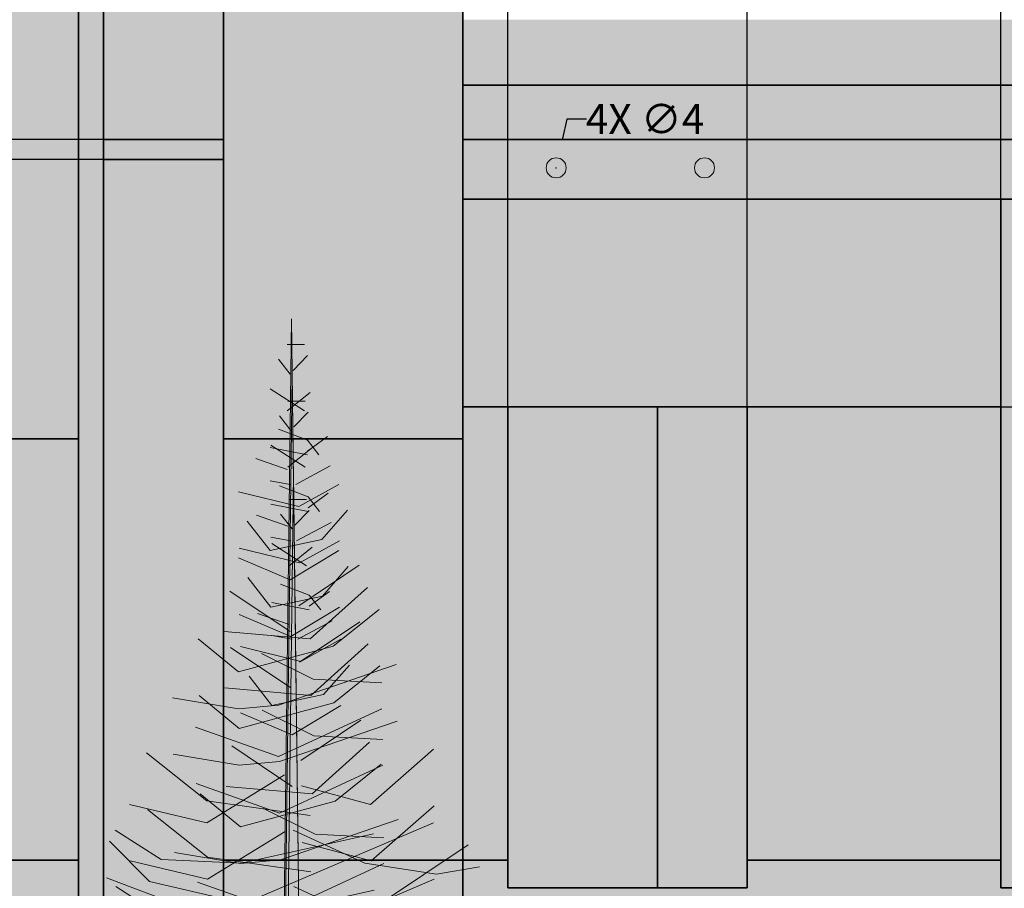
# Model space of a CAD drawing. Units: inches. Extents: x 221 to 874, y 171 to 738.
# Tile 6 of 11: x 452 to 650, y 281 to 455. Entities that reach past the tile are written whole.
import ezdxf

# ---------------------------------------------------------------- set-up
doc = ezdxf.new("R2010")
doc.units = ezdxf.units.IN
doc.header["$MEASUREMENT"] = 0
for name, color, linetype, lineweight in [('A-ANNO-DIMS', 2, 'Continuous', 18), ('A-ELEV', 7, 'Continuous', 35), ('A-ELEV-PATT', 8, 'Continuous', 13), ('E-LITE', 2, 'Continuous', 18), ('L-PLNT', 3, 'Continuous', 13)]:
    doc.layers.add(name, color=color, linetype=linetype, lineweight=lineweight)
doc.styles.get("Standard").update_dxf_attribs({"font": 'arial.ttf'})
doc.dimstyles.get("Standard").update_dxf_attribs({"dimtxt": 6, "dimasz": 4, "dimexe": 0.18, "dimexo": 0.0625, "dimgap": 0.09, "dimtad": 0, "dimtih": 1, "dimtoh": 1, "dimdec": 0, "dimzin": 0, "dimdsep": 46, "dimlunit": 3, "dimtxsty": 'Standard', "dimcen": 0.09, "dimadec": 0, "dimazin": 0, "dimtfac": 1, "dimtdec": 0, "dimtofl": 0, "dimtmove": 0, "dimatfit": 3, "dimfxl": 1, "dimtolj": 1, "dimtzin": 0, "dimarcsym": 0})

# ---------------------------------------------------------------- blocks, each defined once
blk = doc.blocks.new('*D21')
at = {"layer": 'A-ANNO-DIMS', "color": 0, "lineweight": -2, "transparency": 16777216}
for p, q in [((541.14, 706.72), (833.01, 706.72)), ((832.83, 702.72), (832.83, 457.87)), ((832.83, 206.72), (832.83, 451.56)), ((805.14, 202.72), (833.01, 202.72))]:
    blk.add_line(p, q, dxfattribs=at)
at = {"layer": 'A-ANNO-DIMS', "color": 0, "transparency": 16777216}
for points in [[(832.16, 702.72), (833.5, 702.72), (832.83, 706.72)], [(832.16, 206.72), (833.5, 206.72), (832.83, 202.72)]]:
    blk.add_solid(points, dxfattribs=at)
at = {"layer": 'Defpoints', "color": 0, "transparency": 16777216}
for p in [(541.08, 706.72), (832.83, 706.72), (805.08, 202.72)]:
    blk.add_point(p, dxfattribs=at)
at = {"layer": 'A-ANNO-DIMS', "color": 0, "transparency": 16777216, "insert": (832.83, 454.72), "char_height": 6, "attachment_point": 5}
blk.add_mtext('\\A1;504', dxfattribs=at)
blk = doc.blocks.new('*D33')
at = {"layer": 'A-ANNO-DIMS', "color": 0, "lineweight": -2, "transparency": 16777216}
for p, q in [((469.02, 426.72), (231.36, 426.72)), ((231.54, 422.72), (231.54, 401.87)), ((231.54, 374.72), (231.54, 395.56)), ((313.02, 370.72), (231.36, 370.72))]:
    blk.add_line(p, q, dxfattribs=at)
at = {"layer": 'A-ANNO-DIMS', "color": 0, "transparency": 16777216}
for points in [[(230.88, 422.72), (232.21, 422.72), (231.54, 426.72)], [(230.88, 374.72), (232.21, 374.72), (231.54, 370.72)]]:
    blk.add_solid(points, dxfattribs=at)
at = {"layer": 'Defpoints', "color": 0, "transparency": 16777216}
for p in [(231.54, 426.72), (469.08, 426.72), (313.08, 370.72)]:
    blk.add_point(p, dxfattribs=at)
at = {"layer": 'A-ANNO-DIMS', "color": 0, "transparency": 16777216, "insert": (231.54, 398.72), "char_height": 6, "attachment_point": 5}
blk.add_mtext('\\A1;56', dxfattribs=at)
blk = doc.blocks.new('*D34')
at = {"layer": 'A-ANNO-DIMS', "color": 0, "lineweight": -2, "transparency": 16777216}
for p, q in [((231.54, 434.72), (231.54, 438.72)), ((231.54, 438.72), (235.54, 438.72)), ((469.02, 430.72), (231.36, 430.72)), ((469.02, 426.72), (231.36, 426.72)), ((231.54, 422.72), (231.54, 418.72))]:
    blk.add_line(p, q, dxfattribs=at)
at = {"layer": 'A-ANNO-DIMS', "color": 0, "transparency": 16777216}
for points in [[(230.88, 434.72), (232.21, 434.72), (231.54, 430.72)], [(230.88, 422.72), (232.21, 422.72), (231.54, 426.72)]]:
    blk.add_solid(points, dxfattribs=at)
at = {"layer": 'Defpoints', "color": 0, "transparency": 16777216}
for p in [(231.54, 430.72), (469.08, 430.72), (469.08, 426.72)]:
    blk.add_point(p, dxfattribs=at)
at = {"layer": 'A-ANNO-DIMS', "color": 0, "transparency": 16777216, "insert": (237.71, 438.72), "char_height": 6, "attachment_point": 5}
blk.add_mtext('\\A1;4', dxfattribs=at)
blk = doc.blocks.new('*D35')
at = {"layer": 'A-ANNO-DIMS', "color": 0, "lineweight": -2, "transparency": 16777216}
for p, q in [((313.02, 454.72), (231.36, 454.72)), ((231.54, 450.72), (231.54, 445.82)), ((231.54, 434.72), (231.54, 439.61)), ((469.02, 430.72), (231.36, 430.72))]:
    blk.add_line(p, q, dxfattribs=at)
at = {"layer": 'A-ANNO-DIMS', "color": 0, "transparency": 16777216}
for points in [[(230.88, 450.72), (232.21, 450.72), (231.54, 454.72)], [(230.88, 434.72), (232.21, 434.72), (231.54, 430.72)]]:
    blk.add_solid(points, dxfattribs=at)
at = {"layer": 'Defpoints', "color": 0, "transparency": 16777216}
for p in [(231.54, 454.72), (313.08, 454.72), (469.08, 430.72)]:
    blk.add_point(p, dxfattribs=at)
at = {"layer": 'A-ANNO-DIMS', "color": 0, "transparency": 16777216, "insert": (231.54, 442.72), "char_height": 6, "attachment_point": 5}
blk.add_mtext('\\A1;24', dxfattribs=at)
blk = doc.blocks.new('*D57')
at = {"layer": 'A-ANNO-DIMS', "color": 0, "lineweight": -2, "transparency": 16777216}
for p, q in [((541.08, 377.16), (541.08, 734.65)), ((545.08, 734.47), (546.08, 734.47)), ((550.08, 377.16), (550.08, 734.65)), ((550.08, 734.47), (554.08, 734.47))]:
    blk.add_line(p, q, dxfattribs=at)
at = {"layer": 'A-ANNO-DIMS', "color": 0, "transparency": 16777216}
for points in [[(545.08, 735.13), (545.08, 733.8), (541.08, 734.47)], [(546.08, 735.13), (546.08, 733.8), (550.08, 734.47)]]:
    blk.add_solid(points, dxfattribs=at)
at = {"layer": 'Defpoints', "color": 0, "transparency": 16777216}
for p in [(550.08, 734.47), (541.08, 377.1), (550.08, 377.1)]:
    blk.add_point(p, dxfattribs=at)
at = {"layer": 'A-ANNO-DIMS', "color": 0, "transparency": 16777216, "insert": (556.14, 734.47), "char_height": 6, "attachment_point": 5}
blk.add_mtext('\\A1;9', dxfattribs=at)
blk = doc.blocks.new('*D58')
at = {"layer": 'A-ANNO-DIMS', "color": 0, "lineweight": -2, "transparency": 16777216}
for p, q in [((550.08, 377.16), (550.08, 734.65)), ((554.08, 734.47), (569.56, 734.47)), ((594.08, 734.47), (578.59, 734.47)), ((598.08, 377.16), (598.08, 734.65))]:
    blk.add_line(p, q, dxfattribs=at)
at = {"layer": 'A-ANNO-DIMS', "color": 0, "transparency": 16777216}
for points in [[(554.08, 735.13), (554.08, 733.8), (550.08, 734.47)], [(594.08, 735.13), (594.08, 733.8), (598.08, 734.47)]]:
    blk.add_solid(points, dxfattribs=at)
at = {"layer": 'Defpoints', "color": 0, "transparency": 16777216}
for p in [(598.08, 734.47), (550.08, 377.1), (598.08, 377.1)]:
    blk.add_point(p, dxfattribs=at)
at = {"layer": 'A-ANNO-DIMS', "color": 0, "transparency": 16777216, "insert": (574.08, 734.47), "char_height": 6, "attachment_point": 5}
blk.add_mtext('\\A1;48', dxfattribs=at)
blk = doc.blocks.new('*D59')
at = {"layer": 'A-ANNO-DIMS', "color": 0, "lineweight": -2, "transparency": 16777216}
for p, q in [((598.08, 377.16), (598.08, 734.65)), ((602.08, 734.47), (613.28, 734.47)), ((644.91, 734.47), (633.71, 734.47)), ((648.91, 377.16), (648.91, 734.65))]:
    blk.add_line(p, q, dxfattribs=at)
at = {"layer": 'A-ANNO-DIMS', "color": 0, "transparency": 16777216}
for points in [[(602.08, 735.13), (602.08, 733.8), (598.08, 734.47)], [(644.91, 735.13), (644.91, 733.8), (648.91, 734.47)]]:
    blk.add_solid(points, dxfattribs=at)
at = {"layer": 'Defpoints', "color": 0, "transparency": 16777216}
for p in [(648.91, 734.47), (598.08, 377.1), (648.91, 377.1)]:
    blk.add_point(p, dxfattribs=at)
at = {"layer": 'A-ANNO-DIMS', "color": 0, "transparency": 16777216, "insert": (623.49, 734.47), "char_height": 6, "attachment_point": 5}
blk.add_mtext('\\A1;50.83', dxfattribs=at)
blk = doc.blocks.new('*D60')
at = {"layer": 'A-ANNO-DIMS', "color": 0, "lineweight": -2, "transparency": 16777216}
for p, q in [((648.91, 377.16), (648.91, 734.65)), ((652.91, 734.47), (673.02, 734.47)), ((701.91, 734.47), (681.8, 734.47)), ((705.91, 377.16), (705.91, 734.65))]:
    blk.add_line(p, q, dxfattribs=at)
at = {"layer": 'A-ANNO-DIMS', "color": 0, "transparency": 16777216}
for points in [[(652.91, 735.13), (652.91, 733.8), (648.91, 734.47)], [(701.91, 735.13), (701.91, 733.8), (705.91, 734.47)]]:
    blk.add_solid(points, dxfattribs=at)
at = {"layer": 'Defpoints', "color": 0, "transparency": 16777216}
for p in [(705.91, 734.47), (648.91, 377.1), (705.91, 377.1)]:
    blk.add_point(p, dxfattribs=at)
at = {"layer": 'A-ANNO-DIMS', "color": 0, "transparency": 16777216, "insert": (677.41, 734.47), "char_height": 6, "attachment_point": 5}
blk.add_mtext('\\A1;57', dxfattribs=at)
blk = doc.blocks.new('*D65')
at = {"layer": 'A-ANNO-DIMS', "color": 0, "lineweight": -2, "transparency": 16777216}
for p, q in [((598.14, 377.1), (833.01, 377.1)), ((832.83, 373.1), (832.83, 332.06)), ((832.83, 284.72), (832.83, 325.75)), ((705.97, 280.72), (833.01, 280.72))]:
    blk.add_line(p, q, dxfattribs=at)
at = {"layer": 'A-ANNO-DIMS', "color": 0, "transparency": 16777216}
for points in [[(832.16, 373.1), (833.5, 373.1), (832.83, 377.1)], [(832.16, 284.72), (833.5, 284.72), (832.83, 280.72)]]:
    blk.add_solid(points, dxfattribs=at)
at = {"layer": 'Defpoints', "color": 0, "transparency": 16777216}
for p in [(598.08, 377.1), (832.83, 377.1), (705.91, 280.72)]:
    blk.add_point(p, dxfattribs=at)
at = {"layer": 'A-ANNO-DIMS', "color": 0, "transparency": 16777216, "insert": (832.83, 328.91), "char_height": 6, "attachment_point": 5}
blk.add_mtext('\\A1;96.39', dxfattribs=at)
blk = doc.blocks.new('*D66')
at = {"layer": 'A-ANNO-DIMS', "color": 0, "lineweight": -2, "transparency": 16777216}
for p, q in [((781.14, 418.72), (833.01, 418.72)), ((832.83, 414.72), (832.83, 401.06)), ((832.83, 381.1), (832.83, 394.76)), ((598.14, 377.1), (833.01, 377.1))]:
    blk.add_line(p, q, dxfattribs=at)
at = {"layer": 'A-ANNO-DIMS', "color": 0, "transparency": 16777216}
for points in [[(832.16, 414.72), (833.5, 414.72), (832.83, 418.72)], [(832.16, 381.1), (833.5, 381.1), (832.83, 377.1)]]:
    blk.add_solid(points, dxfattribs=at)
at = {"layer": 'Defpoints', "color": 0, "transparency": 16777216}
for p in [(781.08, 418.72), (832.83, 418.72), (598.08, 377.1)]:
    blk.add_point(p, dxfattribs=at)
at = {"layer": 'A-ANNO-DIMS', "color": 0, "transparency": 16777216, "insert": (832.83, 397.91), "char_height": 6, "attachment_point": 5}
blk.add_mtext('\\A1;41.61', dxfattribs=at)
blk = doc.blocks.new('*D68')
at = {"layer": 'A-ANNO-DIMS', "color": 0, "lineweight": -2, "transparency": 16777216}
for p, q in [((231.54, 278.72), (231.54, 282.72)), ((231.54, 282.72), (235.54, 282.72)), ((541.02, 274.72), (231.36, 274.72)), ((541.02, 271.72), (231.36, 271.72)), ((231.54, 267.72), (231.54, 263.72))]:
    blk.add_line(p, q, dxfattribs=at)
at = {"layer": 'A-ANNO-DIMS', "color": 0, "transparency": 16777216}
for points in [[(230.88, 278.72), (232.21, 278.72), (231.54, 274.72)], [(230.88, 267.72), (232.21, 267.72), (231.54, 271.72)]]:
    blk.add_solid(points, dxfattribs=at)
at = {"layer": 'Defpoints', "color": 0, "transparency": 16777216}
for p in [(231.54, 274.72), (541.08, 274.72), (541.08, 271.72)]:
    blk.add_point(p, dxfattribs=at)
at = {"layer": 'A-ANNO-DIMS', "color": 0, "transparency": 16777216, "insert": (237.6, 282.72), "char_height": 6, "attachment_point": 5}
blk.add_mtext('\\A1;3', dxfattribs=at)
blk = doc.blocks.new('*D73')
at = {"layer": 'A-ANNO-DIMS', "color": 0, "lineweight": -2, "transparency": 16777216}
for p, q in [((561.89, 434.8), (561.05, 430.89)), ((565.89, 434.8), (561.89, 434.8)), ((559.7, 425.02), (559.88, 425.02)), ((559.79, 424.93), (559.79, 425.11))]:
    blk.add_line(p, q, dxfattribs=at)
at = {"layer": 'A-ANNO-DIMS', "color": 0, "transparency": 16777216}
blk.add_solid([(560.4, 431.03), (561.7, 430.75), (560.21, 426.98)], dxfattribs=at)
at = {"layer": 'Defpoints', "color": 0, "transparency": 16777216}
for p in [(560.21, 426.98), (559.37, 423.06)]:
    blk.add_point(p, dxfattribs=at)
at = {"layer": 'A-ANNO-DIMS', "color": 0, "transparency": 16777216, "insert": (577.6, 434.8), "char_height": 6, "attachment_point": 5}
blk.add_mtext('\\A1;4X ∅4', dxfattribs=at)

msp = doc.modelspace()

# ---------------------------------------------------------------- hatches: boundary and pattern name
at = {"layer": 'A-ELEV-PATT'}
h = msp.add_hatch(color=256, dxfattribs=at)
h.dxf.hatch_style = 1
h.paths.add_polyline_path([(349.0786, 286.1996), (313.0786, 286.1996), (313.0786, 232.7164), (349.0786, 232.7164)])
h.paths.add_polyline_path([(464.0786, 286.1996), (406.0786, 286.1996), (406.0786, 232.7164), (464.0786, 232.7164)])
h.paths.add_polyline_path([(541.0786, 286.1996), (493.0786, 286.1996), (493.0786, 232.7164), (541.0786, 232.7164)])
h.paths.add_polyline_path([(541.0786, 370.7164), (493.0786, 370.7164), (493.0786, 286.1996), (541.0786, 286.1996)])
h.paths.add_polyline_path([(464.0786, 370.7164), (406.0786, 370.7164), (406.0786, 286.1996), (464.0786, 286.1996)])
h.paths.add_polyline_path([(349.0786, 370.7164), (313.0786, 370.7164), (313.0786, 286.1996), (349.0786, 286.1996)])
h.paths.add_polyline_path([(349.0786, 454.7164), (313.0786, 454.7164), (313.0786, 370.7164), (349.0786, 370.7164)])
h.paths.add_polyline_path([(464.0786, 454.7164), (406.0786, 454.7164), (406.0786, 370.7164), (464.0786, 370.7164)])
h.paths.add_polyline_path([(541.0786, 418.7164), (541.0786, 454.7164), (493.0786, 454.7164), (493.0786, 370.7164), (541.0786, 370.7164)])
h.paths.add_polyline_path([(541.0786, 550.7164), (493.0786, 550.7164), (493.0786, 454.7164), (541.0786, 454.7164)])
h.paths.add_polyline_path([(464.0786, 550.7164), (406.0786, 550.7164), (406.0786, 454.7164), (464.0786, 454.7164)])
h.paths.add_polyline_path([(349.0786, 550.7164), (313.0786, 550.7164), (313.0786, 454.7164), (349.0786, 454.7164)])
h.paths.add_polyline_path([(349.0786, 586.7164), (313.0786, 586.7164), (313.0786, 550.7164), (349.0786, 550.7164)])
h.paths.add_polyline_path([(464.0786, 586.7164), (406.0786, 586.7164), (406.0786, 550.7164), (464.0786, 550.7164)])
h.paths.add_polyline_path([(541.0786, 574.7164), (541.0786, 586.7164), (493.0786, 586.7164), (493.0786, 550.7164), (541.0786, 550.7164)])
h.paths.add_polyline_path([(541.0786, 670.7164), (493.0786, 670.7164), (493.0786, 586.7164), (541.0786, 586.7164)])
h.paths.add_polyline_path([(464.0786, 670.7164), (406.0786, 670.7164), (406.0786, 586.7164), (464.0786, 586.7164)])
h.paths.add_polyline_path([(349.0786, 670.7164), (313.0786, 670.7164), (313.0786, 586.7164), (349.0786, 586.7164)])
h.paths.add_polyline_path([(406.0786, 706.7164), (313.0786, 706.7164), (313.0786, 670.7164), (349.0786, 670.7164), (406.0786, 670.7164)])
h.paths.add_polyline_path([(464.0786, 706.7164), (406.0786, 706.7164), (406.0786, 670.7164), (464.0786, 670.7164)])
h.paths.add_polyline_path([(541.0786, 706.7164), (493.0786, 706.7164), (493.0786, 688.7164), (493.0786, 670.7164), (541.0786, 670.7164)])
h.paths.add_polyline_path([(660.0786, 610.7164), (541.0786, 610.7164), (541.0786, 586.7164), (541.0786, 574.7164), (660.0786, 574.7164)])
h.paths.add_polyline_path([(781.0786, 610.7164), (660.0786, 610.7164), (660.0786, 574.7164), (769.0786, 574.7164), (781.0786, 574.7164)])
h.paths.add_polyline_path([(781.0786, 574.7164), (769.0786, 574.7164), (769.0786, 476.1199), (781.0786, 476.1199)])
h.paths.add_polyline_path([(781.0786, 476.1199), (769.0786, 476.1199), (769.0786, 457.7164), (781.0786, 457.7164)])
h.paths.add_polyline_path([(781.0786, 377.1023), (705.9097, 377.1023), (705.9097, 286.1996), (781.0786, 286.1996)])
h.paths.add_polyline_path([(741.9618, 338.8486), (756.9618, 338.8486), (756.9618, 329.8486), (741.9618, 329.8486)], flags=16)
h.paths.add_polyline_path([(648.9097, 377.1023), (598.0786, 377.1023), (598.0786, 286.1996), (648.9097, 286.1996)])
h.paths.add_polyline_path([(781.0786, 286.1996), (705.9097, 286.1996), (705.9097, 280.7164), (648.9097, 280.7164), (648.9097, 286.1996), (598.0786, 286.1996), (598.0786, 280.7164), (550.0786, 280.7164), (550.0786, 286.1996), (541.0786, 286.1996), (541.0786, 274.7164), (781.0786, 274.7164)])
h.paths.add_polyline_path([(660.0786, 562.7164), (546.3477, 562.7164), (546.3477, 457.7164), (660.0786, 457.7164)])
h = msp.add_hatch(color=256, dxfattribs=at)
h.set_gradient(color1=(255, 236, 199), name='CYLINDER')
h.paths.add_polyline_path([(469.0786, 680.7164), (464.0786, 680.7164), (464.0786, 232.7164), (469.0786, 232.7164)])
h = msp.add_hatch(color=256, dxfattribs=at)
h.set_gradient(color1=(147, 149, 152), color2=(254, 234, 185), name='CYLINDER')
h.paths.add_polyline_path([(469.0786, 430.7164), (493.0786, 430.7164), (493.0786, 680.7164), (469.0786, 680.7164)])
h = msp.add_hatch(color=256, dxfattribs=at)
h.dxf.hatch_style = 1
h.paths.add_polyline_path([(793.0786, 441.595), (793.0786, 454.7164), (541.0786, 454.7164), (541.0786, 441.595)])
h = msp.add_hatch(color=256, dxfattribs=at)
h.dxf.hatch_style = 1
h.paths.add_polyline_path([(793.0786, 430.7164), (793.0786, 441.595), (541.0786, 441.595), (541.0786, 430.7164)])
for points in [[(493.0786, 430.7164), (469.0786, 430.7164), (469.0786, 426.7164), (493.0786, 426.7164)], [(580.0786, 377.1023), (550.0786, 377.1023), (550.0786, 280.7164), (580.0786, 280.7164)], [(580.0786, 280.7164), (598.0786, 280.7164), (598.0786, 377.1023), (580.0786, 377.1023)]]:
    msp.add_hatch(color=256, dxfattribs=at).paths.add_polyline_path(points)
h = msp.add_hatch(color=256, dxfattribs=at)
h.set_gradient(color1=(209, 204, 163), color2=(147, 149, 152), rotation=90, name='INVCYLINDER')
h.paths.add_polyline_path([(781.0786, 418.7164), (793.0786, 430.7164), (541.0786, 430.7164), (541.0786, 418.7164)])
h.paths.add_polyline_path([(587.5133, 425.0196, -1), (591.5133, 425.0196, -1)], flags=16)
h.paths.add_polyline_path([(557.7898, 425.0196, -1), (561.7898, 425.0196, -1)], flags=16)
h = msp.add_hatch(color=256, dxfattribs=at)
h.set_gradient(color1=(99, 100, 102), color2=(254, 234, 185), name='INVCYLINDER')
h.paths.add_polyline_path([(493.0786, 426.7164), (469.0786, 426.7164), (469.0786, 232.7164), (493.0786, 232.7164)])
h = msp.add_hatch(color=256, dxfattribs=at)
h.paths.add_polyline_path([(561.7898, 425.0196, 1), (557.7898, 425.0196, 1)])
h.paths.add_polyline_path([(591.5133, 425.0196, 1), (587.5133, 425.0196, 1)])
h = msp.add_hatch(color=256, dxfattribs=at)
h.set_gradient(color1=(209, 204, 163), color2=(80, 81, 83), rotation=90)
h.paths.add_polyline_path([(541.0786, 418.7164), (541.0786, 377.1023), (550.0786, 377.1023), (598.0786, 377.1023), (648.9097, 377.1023), (648.9097, 418.7164)])
h = msp.add_hatch(color=256, dxfattribs=at)
h.paths.add_polyline_path([(705.9097, 418.7164), (648.9097, 418.7164), (648.9097, 280.7164), (705.9097, 280.7164)])
h.paths.add_polyline_path([(675.9097, 415.7164), (675.9097, 283.7164), (651.9097, 283.7164), (651.9097, 415.7164)], flags=16)
h.paths.add_polyline_path([(678.9097, 415.7164), (702.9097, 415.7164), (702.9097, 283.7164), (678.9097, 283.7164)], flags=16)
h = msp.add_hatch(color=256, dxfattribs=at)
h.set_gradient(color1=(80, 81, 83), color2=(179, 180, 121))
h.paths.add_polyline_path([(541.0786, 286.1996), (550.0786, 286.1996), (550.0786, 377.1023), (541.0786, 377.1023)])

# ---------------------------------------------------------------- linework, layer by layer
at = {"layer": 'A-ELEV'}
for p, q in [((464.0786, 706.7164), (464.0786, 232.7164)), ((493.0786, 688.7164), (493.0786, 232.7164)), ((469.0786, 684.7164), (469.0786, 232.7164)), ((541.0786, 418.7164), (541.0786, 574.7164)), ((541.0786, 441.595), (793.0786, 441.595)), ((493.0786, 430.7164), (469.0786, 430.7164)), ((793.0786, 430.7164), (541.0786, 430.7164)), ((493.0786, 426.7164), (469.0786, 426.7164)), ((781.0786, 418.7164), (541.0786, 418.7164)), ((541.0786, 418.7164), (541.0786, 228.7164)), ((648.9097, 418.7164), (648.9097, 280.7164)), ((550.0786, 377.1023), (541.0786, 377.1023)), ((550.0786, 377.1023), (550.0786, 280.7164)), ((598.0786, 377.1023), (550.0786, 377.1023)), ((580.0786, 280.7164), (580.0786, 377.1023)), ((598.0786, 280.7164), (598.0786, 377.1023)), ((598.0786, 377.1023), (648.9097, 377.1023)), ((406.0786, 370.7164), (464.0786, 370.7164)), ((493.0786, 370.7164), (541.0786, 370.7164)), ((406.0786, 286.1996), (464.0786, 286.1996)), ((493.0786, 286.1996), (541.0786, 286.1996)), ((541.0786, 286.1996), (550.0786, 286.1996)), ((598.0786, 286.1996), (648.9097, 286.1996)), ((550.0786, 280.7164), (598.0786, 280.7164)), ((705.9097, 280.7164), (648.9097, 280.7164))]:
    msp.add_line(p, q, dxfattribs=at)
msp.add_lwpolyline([(464.0786, 680.7164), (469.0786, 680.7164), (469.0786, 232.7164), (464.0786, 232.7164)], close=True, dxfattribs=at)
at = {"layer": 'E-LITE'}
for centre in [(559.7898, 425.0196), (589.5133, 425.0196)]:
    msp.add_circle(centre, 2, dxfattribs=at)
at = {"layer": 'L-PLNT'}
for p, q in [((506.7539, 394.7164), (504.3549, 202.7164)), ((506.7539, 394.7164), (509.1549, 202.7164)), ((505.8919, 389.5854), (509.3429, 389.5854)), ((507.0419, 384.4244), (509.9179, 387.3734)), ((504.1669, 386.6364), (506.4669, 383.6874)), ((506.8956, 383.3859), (504.6382, 202.7164)), ((506.8956, 383.3859), (509.1549, 202.7164)), ((502.4409, 380.7384), (509.3429, 376.3144)), ((505.8919, 376.3144), (510.4929, 380.0004)), ((506.0336, 378.2549), (509.4846, 378.2549)), ((504.3086, 375.3059), (506.6086, 372.3569)), ((507.1836, 373.0939), (510.0596, 376.0429)), ((504.1669, 372.6274), (509.9179, 370.4154)), ((509.9179, 368.2034), (513.9429, 371.1534)), ((502.5826, 369.4079), (509.4846, 364.9839)), ((509.9179, 370.4154), (512.2179, 367.4664)), ((502.4409, 368.9414), (509.9179, 367.4664)), ((506.0336, 364.9839), (510.6346, 368.6699)), ((505.8919, 364.5174), (499.5649, 366.7294)), ((507.6169, 361.5684), (514.5189, 365.2544)), ((507.1423, 363.6628), (505.1313, 202.7164)), ((507.1423, 363.6628), (509.1549, 202.7164)), ((502.4409, 362.3054), (506.4669, 361.5684)), ((504.3086, 361.2969), (510.0596, 359.0849)), ((516.2439, 361.5684), (508.1919, 357.1444)), ((508.1919, 357.1444), (496.1149, 360.0934)), ((510.0596, 356.8729), (514.0846, 359.8229)), ((502.5826, 357.6109), (510.0596, 356.1359)), ((506.2803, 358.5318), (509.7313, 358.5318)), ((510.0596, 359.0849), (512.3596, 356.1359)), ((506.0336, 353.1869), (499.7066, 355.3989)), ((504.5553, 355.5828), (506.8553, 352.6338)), ((507.4303, 353.3708), (510.3063, 356.3198)), ((507.7586, 350.2379), (514.6606, 353.9239)), ((502.5826, 350.9749), (506.6086, 350.2379)), ((502.8293, 349.6848), (509.7313, 345.2608)), ((516.3856, 350.2379), (508.3336, 345.8139)), ((508.3336, 345.8139), (496.2566, 348.7629)), ((506.2803, 345.2608), (510.8813, 348.9468)), ((504.5553, 341.5738), (510.3063, 339.3618)), ((510.3063, 337.1498), (514.3313, 340.0998)), ((502.8293, 337.8878), (510.3063, 336.4128)), ((510.3063, 339.3618), (512.6063, 336.4128)), ((506.2803, 333.4638), (499.9533, 335.6758)), ((508.0053, 330.5148), (514.9073, 334.2008)), ((502.8293, 331.2518), (506.8553, 330.5148)), ((516.6323, 330.5148), (508.5803, 326.0908)), ((508.5803, 326.0908), (496.5033, 329.0398))]:
    msp.add_line(p, q, dxfattribs=at)
for points in [[(517.9689, 356.4074), (512.7929, 350.5084), (502.4409, 348.2964), (497.8399, 354.1954)], [(496.1149, 346.8224), (506.4669, 342.3984), (516.2439, 348.2964)], [(508.1919, 337.2374), (520.2699, 345.3474)], [(518.1106, 345.0769), (512.9346, 339.1779), (502.5826, 336.9659), (497.9816, 342.8649)], [(493.2389, 332.0764), (510.4929, 330.6014), (521.9949, 340.9234)], [(494.3889, 340.1864), (506.4669, 332.0764)], [(488.0629, 330.6014), (496.1149, 323.9654), (515.0939, 329.1264), (524.2959, 336.4994)], [(496.2566, 335.4919), (506.6086, 331.0679), (516.3856, 336.9659)], [(508.3336, 325.9069), (520.4116, 334.0169)], [(493.3806, 320.7459), (510.6346, 319.2709), (522.1366, 329.5929)], [(494.5306, 328.8559), (506.6086, 320.7459)], [(500.7159, 327.6524), (511.0679, 322.4914), (524.8709, 321.7534)], [(482.8869, 318.8044), (496.1149, 316.5924), (504.1669, 317.3294), (527.7459, 325.4404)], [(488.2046, 319.2709), (496.2566, 312.6349), (515.2356, 317.7959), (524.4376, 325.1689)], [(518.3573, 325.3538), (513.1813, 319.4548), (502.8293, 317.2428), (498.2283, 323.1418)], [(487.4879, 312.9064), (504.1669, 307.0074), (524.8709, 316.5924)], [(496.5033, 315.7688), (506.8553, 311.3448), (516.6323, 317.2428)], [(500.8576, 316.3219), (511.2096, 311.1609), (525.0126, 310.4229)], [(483.0286, 307.4739), (496.2566, 305.2619), (504.3086, 305.9989), (527.8876, 314.1099)], [(508.5803, 306.1838), (520.6583, 314.2938)], [(493.6273, 301.0228), (510.8813, 299.5478), (522.3833, 309.8698)], [(494.7773, 309.1328), (506.8553, 301.0228)], [(508.7669, 301.1094), (522.5699, 297.4224), (535.2229, 308.4824)], [(477.7109, 307.7444), (489.7889, 298.1594), (510.4929, 295.2104)], [(487.6296, 301.5759), (504.3086, 295.6769), (525.0126, 305.2619)], [(488.4513, 299.5478), (496.5033, 292.9118), (515.4823, 298.0728), (524.6843, 305.4458)], [(474.2599, 297.4224), (489.7889, 293.7364), (505.3169, 303.3214)], [(477.8526, 296.4139), (489.9306, 286.8289), (510.6346, 283.8799)], [(501.1043, 296.5988), (511.4563, 291.4378), (525.2593, 290.6998)], [(508.9086, 289.7789), (522.7116, 286.0919), (535.3646, 297.1519)], [(483.2753, 287.7508), (496.5033, 285.5388), (504.5553, 286.2758), (528.1343, 294.3868)], [(470.2349, 290.0494), (478.2859, 281.9394), (497.2649, 277.5154), (535.2229, 293.7364)], [(471.3849, 292.2614), (480.5869, 286.3634), (496.6899, 285.6254), (523.1449, 291.5244)], [(507.0419, 292.2614), (521.4199, 285.6254), (535.7979, 283.4134), (544.4249, 284.8884)], [(474.4016, 286.0919), (489.9306, 282.4059), (505.4586, 291.9909)], [(469.6589, 282.6764), (498.9899, 271.6174), (515.6689, 271.6174), (542.1239, 289.3124)], [(487.8763, 281.8528), (504.5553, 275.9538), (525.2593, 285.5388)], [(470.3766, 278.7189), (478.4276, 270.6089), (497.4066, 266.1849), (535.3646, 282.4059)], [(471.5266, 280.9309), (480.7286, 275.0329), (496.8316, 274.2949), (523.2866, 280.1939)], [(507.1836, 280.9309), (521.5616, 274.2949), (535.9396, 272.0829), (544.5666, 273.5579)]]:
    msp.add_lwpolyline(points, dxfattribs=at)

# ---------------------------------------------------------------- dimensions: what is measured, and where the dimension line sits
at = {"layer": 'A-ANNO-DIMS'}
for base, p1, p2, override, picture, middle in [((550.0786, 734.4664), (541.0786, 377.1023), (550.0786, 377.1023), {"dimdec": 0, "dimlfac": 1, "dimrnd": 0, "dimzin": 0, "dimdsep": 46, "dimlunit": 2}, '*D57', (556.1413, 734.4664)), ((598.0786, 734.4664), (550.0786, 377.1023), (598.0786, 377.1023), {"dimdec": 0, "dimlfac": 1, "dimrnd": 0, "dimzin": 0, "dimdsep": 46, "dimlunit": 2}, '*D58', (574.0786, 734.4664)), ((648.9097, 734.4664), (598.0786, 377.1023), (648.9097, 377.1023), {"dimdec": 2, "dimlfac": 1, "dimrnd": 0, "dimzin": 0, "dimdsep": 46, "dimlunit": 2}, '*D59', (623.4941, 734.4664)), ((705.9097, 734.4664), (648.9097, 377.1023), (705.9097, 377.1023), {"dimdec": 0, "dimlfac": 1, "dimrnd": 0, "dimzin": 0, "dimdsep": 46, "dimlunit": 2}, '*D60', (677.4097, 734.4664))]:
    dim = msp.add_linear_dim(base=base, p1=p1, p2=p2, dimstyle='Standard', override=override, dxfattribs=at)
    dim.commit()
    dim.dimension.update_dxf_attribs({"geometry": picture, "text_midpoint": middle})
for base, p1, p2, override, picture, middle in [((832.8286, 706.7164), (805.0786, 202.7164), (541.0786, 706.7164), {"dimdec": 0, "dimlfac": 1, "dimrnd": 0, "dimzin": 0, "dimdsep": 46, "dimlunit": 2}, '*D21', (832.8286, 454.7164)), ((231.5426, 454.7164), (469.0786, 430.7164), (313.0786, 454.7164), {"dimdec": 0, "dimlfac": 1, "dimrnd": 0, "dimzin": 0, "dimdsep": 46, "dimlunit": 2}, '*D35', (231.5426, 442.7164)), ((231.5426, 430.7164), (469.0786, 426.7164), (469.0786, 430.7164), {"dimdec": 0, "dimlfac": 1, "dimrnd": 0, "dimzin": 0, "dimdsep": 46, "dimlunit": 2}, '*D34', (237.7077, 438.7164)), ((231.5426, 426.7164), (313.0786, 370.7164), (469.0786, 426.7164), {"dimdec": 0, "dimlfac": 1, "dimrnd": 0, "dimzin": 0, "dimdsep": 46, "dimlunit": 2}, '*D33', (231.5426, 398.7164)), ((832.8286, 418.7164), (598.0786, 377.1023), (781.0786, 418.7164), {"dimdec": 2, "dimlfac": 1, "dimrnd": 0, "dimzin": 0, "dimdsep": 46, "dimlunit": 2}, '*D66', (832.8286, 397.9093)), ((832.8286, 377.1023), (705.9097, 280.7164), (598.0786, 377.1023), {"dimdec": 2, "dimlfac": 1, "dimrnd": 0, "dimzin": 0, "dimdsep": 46, "dimlunit": 2}, '*D65', (832.8286, 328.9093)), ((231.5426, 274.7164), (541.0786, 271.7164), (541.0786, 274.7164), {"dimdec": 0, "dimlfac": 1, "dimrnd": 0, "dimzin": 0, "dimdsep": 46, "dimlunit": 2}, '*D68', (237.5972, 282.7164))]:
    dim = msp.add_linear_dim(base=base, p1=p1, p2=p2, angle=90, dimstyle='Standard', override=override, dxfattribs=at)
    dim.commit()
    dim.dimension.update_dxf_attribs({"geometry": picture, "text_midpoint": middle})
dim = msp.add_diameter_dim_2p(p1=(559.3704, 423.0641), p2=(560.2091, 426.9751), text='4X <>', dimstyle='Standard', override={"dimdec": 0, "dimlfac": 1, "dimrnd": 0, "dimzin": 0, "dimdsep": 46, "dimlunit": 2}, dxfattribs=at)
dim.commit()
dim.dimension.update_dxf_attribs({"geometry": '*D73', "text_midpoint": (577.602, 434.7973), "dimtype": 163})

doc.saveas('drawing.dxf')
